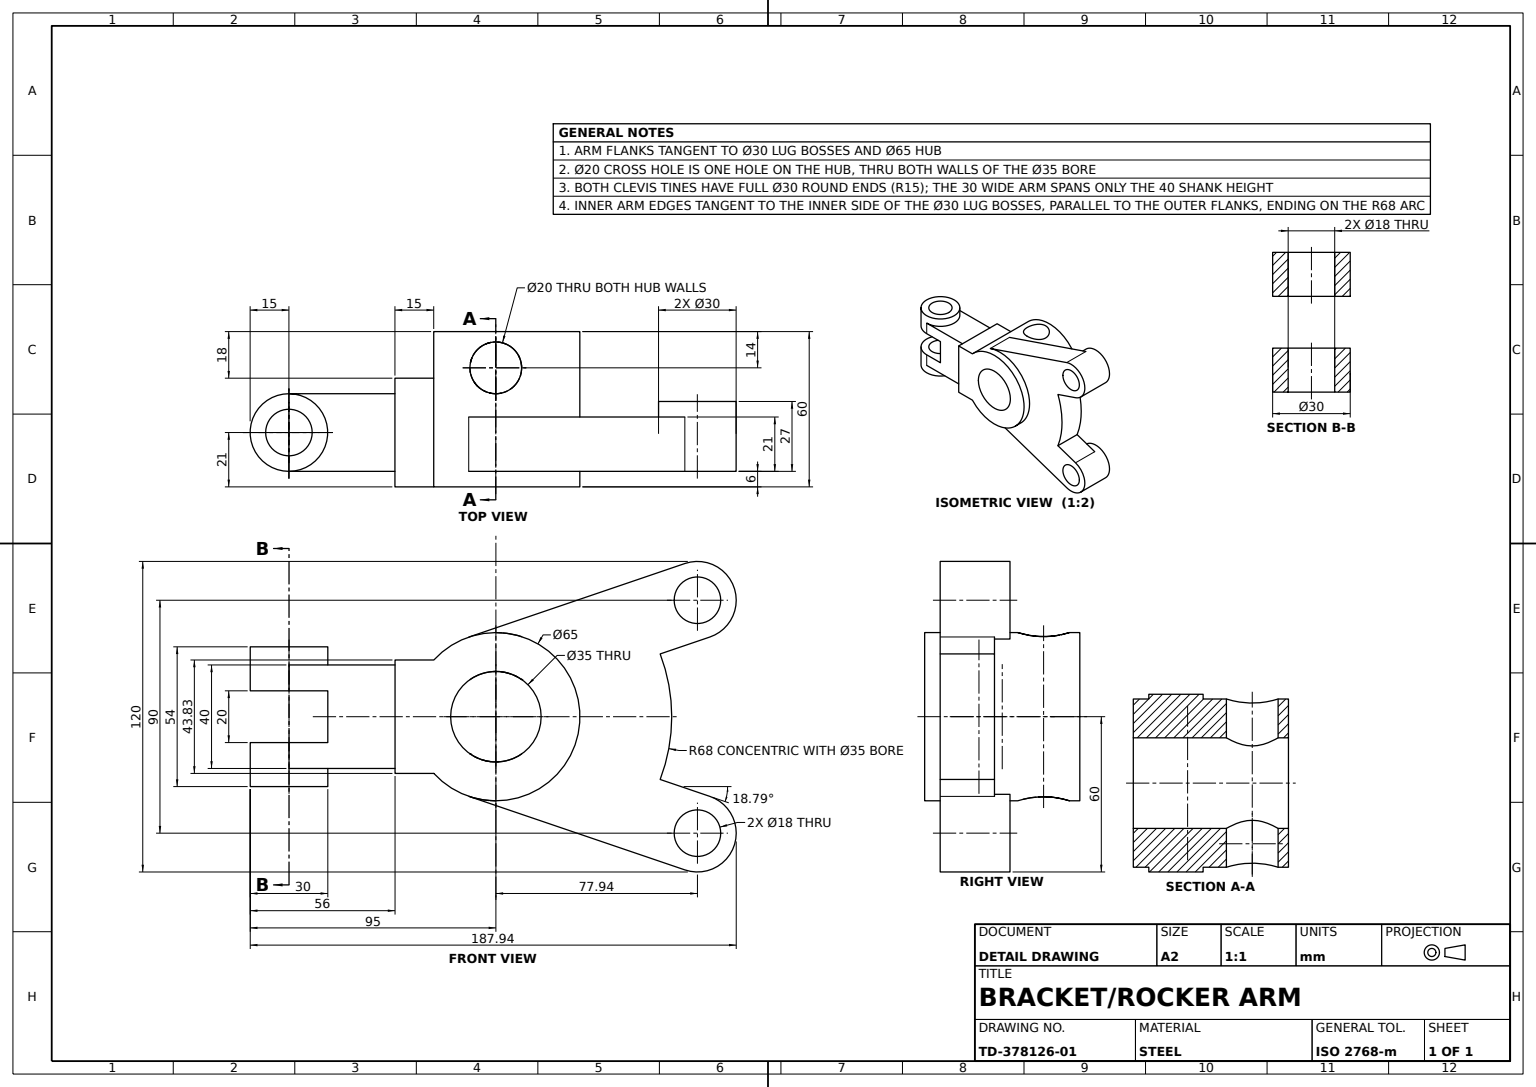
from build123d import *

# Parameters (mm, degrees)
HUB_SKETCH_R                 = 32.5
HUB_SKETCH_R_2               = 17.5
HUB_BOSS_65_DEPTH            = 30
ARM_WEB_DEPTH                = 21
SKETCH3_3_R                  = 15
SKETCH3_3_R_2                = 9
ARM_END_LUGS_DEPTH           = 27
CROSS_HOLE_SKETCH_R          = 10
CROSS_HOLE_14_DEPTH          = 48
CLEVIS_BLOCK_SKETCH_W        = 56
CLEVIS_BLOCK_SKETCH_H        = 40
CLEVIS_BLOCK_DEPTH           = 30
REAR_BOSS_SKETCH_W           = 15
REAR_BOSS_SKETCH_H           = 43.829214002
REAR_BOSS_DEPTH              = 42
CLEVIS_ARM_SKETCH_W          = 15
CLEVIS_ARM_SKETCH_H          = 10
CLEVIS_ARM_DEPTH             = 30
CLEVIS_SLOT_DEPTH            = 118.987287481
CLEVIS_SLOT_DEPTH_BACK       = 42
SKETCH8_3_W                  = 15
SKETCH8_3_H                  = 20
CLEVIS_PIN_HOLE_SKETCH_R     = 9
CLEVIS_PIN_HOLE_18_DEPTH     = 90
CLEVIS_RECESS_DEPTH          = 7
CLEVIS_BLOCK_FILLET_A_RADIUS = 15
CLEVIS_BLOCK_FILLET_A_LENGTH = 17
CLEVIS_BLOCK_FILLET_B_RADIUS = 15
CLEVIS_BLOCK_FILLET_B_LENGTH = 17
REAR_START                   = -18
REAR_BOSS_CUT_DEPTH          = 18


with BuildPart() as part:
    # Hub Sketch → Hub Boss _65 (new, symmetric)
    with BuildSketch(Plane.XY):
        Circle(HUB_SKETCH_R)
        Circle(HUB_SKETCH_R_2, mode=Mode.SUBTRACT)
    extrude(amount=HUB_BOSS_65_DEPTH, both=True)

    # Arm Profile Sketch → Arm Web (add)
    with BuildSketch(Plane.XY.offset(24)):
        with BuildLine():
            Line((63.528162364, 24.252269722), (82.77322949, 30.799225786))
            ThreePointArc((82.77322949, 30.799225786), (63.741512282, 40.169056393), (73.111342275, 59.200773903))
            Line((73.111342275, 59.200773903), (-10.467045475, 30.768343456))
            ThreePointArc((-10.467045475, 30.768343456), (18.921826313, 26.423748579), (32.5, 0))
            ThreePointArc((32.5, 0), (18.921826313, -26.423748579), (-10.467045475, -30.768343456))
            Line((-10.467045475, -30.768343456), (73.111342275, -59.200773903))
            ThreePointArc((73.111342275, -59.200773903), (63.741512551, -40.169055602), (82.773231072, -30.799226324))
            Line((82.773231072, -30.799226324), (63.528162364, -24.252269722))
            ThreePointArc((63.528162364, -24.252269722), (68, 0), (63.528162364, 24.252269722))
        make_face()
    extrude(amount=-ARM_WEB_DEPTH)

    # Sketch3_3 → Arm End Lugs (add)
    # profile 1 of 2: a face of its own
    with BuildSketch(Plane.XY.offset(24)):
        with Locations((77.942286341, 45)):
            Circle(SKETCH3_3_R)
        with Locations((77.942286341, 45)):
            Circle(SKETCH3_3_R_2, mode=Mode.SUBTRACT)
    # profile 2 of 2: a face of its own
    with BuildSketch(Plane.XY.offset(24)):
        with Locations((77.942286341, -45)):
            Circle(SKETCH3_3_R)
        with Locations((77.942286341, -45)):
            Circle(SKETCH3_3_R_2, mode=Mode.SUBTRACT)
    extrude(amount=-ARM_END_LUGS_DEPTH)

    # Cross Hole Sketch → Cross Hole _14 (cut, symmetric)
    with BuildSketch(Plane(origin=(0, 0, 0), x_dir=(1, 0, 0), z_dir=(0, 1, 0))):
        with Locations(Location((0, 16, 0), (0, 0, 270))):
            Circle(CROSS_HOLE_SKETCH_R)
    extrude(amount=CROSS_HOLE_14_DEPTH, both=True, mode=Mode.SUBTRACT)

    # Clevis Block Sketch → Clevis Block (add)
    with BuildSketch(Plane.XY.offset(24)):
        with Locations((-52, 0)):
            Rectangle(CLEVIS_BLOCK_SKETCH_W, CLEVIS_BLOCK_SKETCH_H)
    extrude(amount=-CLEVIS_BLOCK_DEPTH)

    # Rear Boss Sketch → Rear Boss (add)
    with BuildSketch(Plane.XY.offset(30)):
        with Locations((-31.5, 0)):
            Rectangle(REAR_BOSS_SKETCH_W, REAR_BOSS_SKETCH_H)
    extrude(amount=-REAR_BOSS_DEPTH)

    # Clevis Arm Sketch → Clevis Arm (add)
    with BuildSketch(Plane(origin=(0, 0, -6), x_dir=(-1, 0, 0), z_dir=(0, 0, -1))):
        Polygon((80, 20), (80, 10), (95, 10), (95, 27), (65, 27), (65, 20), align=None)
        with Locations((72.5, 15)):
            Rectangle(CLEVIS_ARM_SKETCH_W, CLEVIS_ARM_SKETCH_H)
        Polygon((65, -27), (95, -27), (95, -10), (80, -10), (80, -20), (65, -20), align=None)
        with Locations((72.5, -15)):
            Rectangle(CLEVIS_ARM_SKETCH_W, CLEVIS_ARM_SKETCH_H)
    extrude(amount=-CLEVIS_ARM_DEPTH)

    # Sketch8_3 → Clevis Slot (cut, two sides: drawn at the far end of the back side and taken through both)
    with BuildSketch(Plane(origin=(0, 0, -6), x_dir=(-1, 0, 0), z_dir=(0, 0, -1)).offset(-CLEVIS_SLOT_DEPTH_BACK)):
        with Locations((72.5, 0)):
            Rectangle(SKETCH8_3_W, SKETCH8_3_H)
    extrude(amount=CLEVIS_SLOT_DEPTH + CLEVIS_SLOT_DEPTH_BACK, mode=Mode.SUBTRACT)

    # Clevis Pin Hole Sketch → Clevis Pin Hole _18 (cut)
    with BuildSketch(Plane(origin=(0, 27, 0), x_dir=(1, 0, 0), z_dir=(0, 1, 0))):
        with Locations(Location((-80, -9, 0), (0, 0, 180))):
            Circle(CLEVIS_PIN_HOLE_SKETCH_R)
    extrude(amount=-CLEVIS_PIN_HOLE_18_DEPTH, mode=Mode.SUBTRACT)

    # Clevis Recess Sketch → Clevis Recess (cut)
    with BuildSketch(Plane(origin=(0, 27, 0), x_dir=(1, 0, 0), z_dir=(0, 1, 0))):
        with BuildLine():
            ThreePointArc((-80, 6), (-69.393398282, 1.606601718), (-65, -9))
            Line((-65, -9), (-65, 6))
            Line((-65, 6), (-80, 6))
        make_face()
        with BuildLine():
            Line((-80, -24), (-65, -24))
            Line((-65, -24), (-65, -9))
            ThreePointArc((-65, -9), (-69.393398282, -19.606601718), (-80, -24))
        make_face()
    clevis_recess = extrude(amount=-CLEVIS_RECESS_DEPTH, mode=Mode.SUBTRACT)

    # Clevis Recess Mirror: Clevis Recess across plane
    add(clevis_recess.mirror(Plane.ZX), mode=Mode.SUBTRACT)

    # Clevis Block Fillet A: full round fillet: the end face becomes a half cylinder, R = half its width
    clevis_block_fillet_a_face = Plane((-95, 18.5, 9), x_dir=(0, -1, 0), z_dir=(-1, 0, 0))  # on the end face: x along it, z out of the body
    clevis_block_fillet_a_slab = clevis_block_fillet_a_face.offset(-CLEVIS_BLOCK_FILLET_A_RADIUS / 2) * Box(CLEVIS_BLOCK_FILLET_A_LENGTH, 2 * CLEVIS_BLOCK_FILLET_A_RADIUS, CLEVIS_BLOCK_FILLET_A_RADIUS, mode=Mode.PRIVATE)  # the body's end, R deep
    clevis_block_fillet_a_round = Plane((-80, 18.5, 9), x_dir=(-1, 0, 0), z_dir=(0, -1, 0)) * Cylinder(CLEVIS_BLOCK_FILLET_A_RADIUS, CLEVIS_BLOCK_FILLET_A_LENGTH, mode=Mode.PRIVATE)  # its axis R under the face
    add(clevis_block_fillet_a_slab - clevis_block_fillet_a_round, mode=Mode.SUBTRACT)

    # Clevis Block Fillet B: full round fillet: the end face becomes a half cylinder, R = half its width
    clevis_block_fillet_b_face = Plane((-95, -18.5, 9), x_dir=(0, 1, 0), z_dir=(-1, 0, 0))  # on the end face: x along it, z out of the body
    clevis_block_fillet_b_slab = clevis_block_fillet_b_face.offset(-CLEVIS_BLOCK_FILLET_B_RADIUS / 2) * Box(CLEVIS_BLOCK_FILLET_B_LENGTH, 2 * CLEVIS_BLOCK_FILLET_B_RADIUS, CLEVIS_BLOCK_FILLET_B_RADIUS, mode=Mode.PRIVATE)  # the body's end, R deep
    clevis_block_fillet_b_round = Plane((-80, -18.5, 9), x_dir=(-1, 0, 0), z_dir=(0, 1, 0)) * Cylinder(CLEVIS_BLOCK_FILLET_B_RADIUS, CLEVIS_BLOCK_FILLET_B_LENGTH, mode=Mode.PRIVATE)  # its axis R under the face
    add(clevis_block_fillet_b_slab - clevis_block_fillet_b_round, mode=Mode.SUBTRACT)

    # Rear Boss Cut Sketch → Rear Boss Cut (cut)
    with BuildSketch(Plane(origin=(0, 0, -30), x_dir=(-1, 0, 0), z_dir=(0, 0, -1)).offset(REAR_START)):
        with BuildLine():
            Line((24, 21.914607001), (24, -21.914607001))
            ThreePointArc((24, -21.914607001), (32.5, 0), (24, 21.914607001))
        make_face()
    extrude(amount=REAR_BOSS_CUT_DEPTH, mode=Mode.SUBTRACT)


solid = part.part
